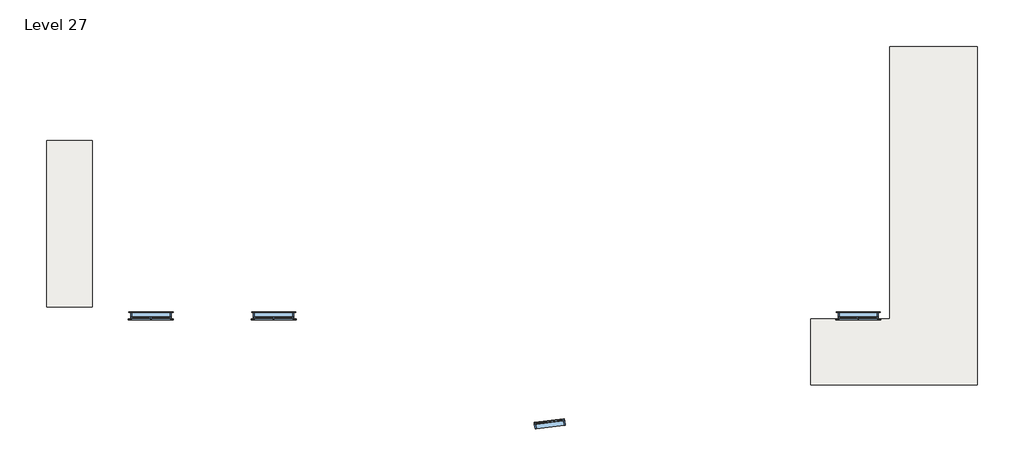
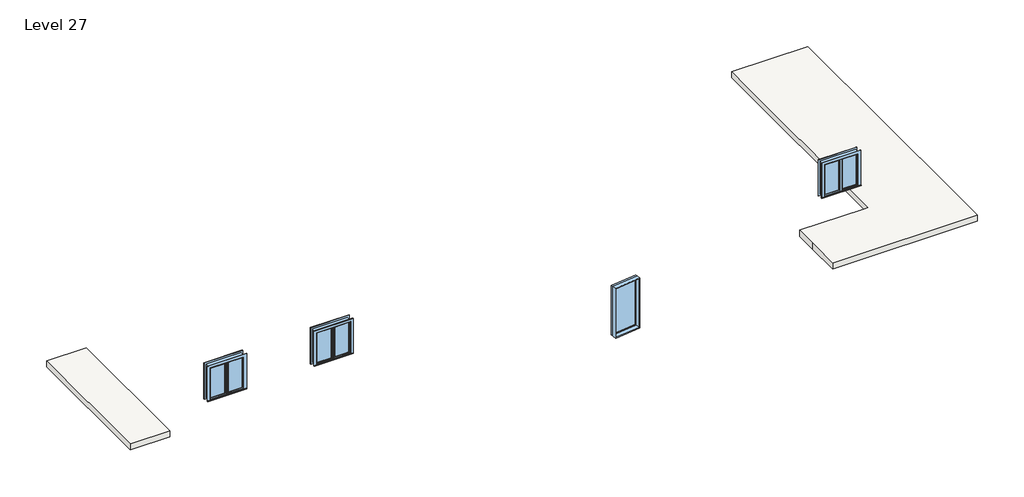
# One storey: 4 windows, 2 slabs.
"""IFC4 building model written with IfcOpenShell, lengths in millimetres."""

from ifc_helpers import new_model, si_unit, frame, origin, place, context, project, spatial, polyline, outline, extrude, transform, mapped, element, save
from components import window_0862ab64, window_9a779fa2

model = new_model("IFC4")

# Units and contexts
model_context = context("Model", 3, world=origin())
ifc_project = project(units=[si_unit("LENGTHUNIT", "METRE", prefix="MILLI")], contexts=[model_context])

# Site, building, storey
site = spatial("IfcSite", under=ifc_project)
building = spatial("IfcBuilding", under=site)
storey = spatial("IfcBuildingStorey", under=building, Name="Level 27", Elevation=42595.8)

# Slabs
placement = place(None, origin())
element("IfcSlab", 1, ObjectType="9\"", at=placement, inside=storey, context=model_context, shape_type="SweptSolid", body=[
    extrude(outline(polyline([(-17978.526008, -8690.0239591), (-16606.926008, -8690.0239591), (-16606.926008, -13719.2239591), (-17978.526008, -13719.2239591), (-17978.526008, -8690.0239591)])), frame((0.0, 0.0, 42367.2), z_axis=(0.0, 0.0, 1.0), x_axis=(1.0, 0.0, 0.0)), (0.0, 0.0, 1.0), 228.6),
])
element("IfcSlab", 2, ObjectType="9\"", at=placement, inside=storey, context=model_context, shape_type="SweptSolid", body=[
    extrude(outline(polyline([(5071.4396352, -14840.0808221), (5071.4396352, -14078.0808221), (7255.8396352, -14078.0808221), (7459.0396352, -14078.0808221), (7459.0396352, -5848.4808221), (10100.6396352, -5848.4808221), (10100.6396352, -14840.0808221), (10100.6396352, -16059.2808221), (5071.4396352, -16059.2808221), (5071.4396352, -14840.0808221)])), frame((0.0, 0.0, 42367.2), z_axis=(0.0, 0.0, 1.0), x_axis=(1.0, 0.0, 0.0)), (0.0, 0.0, 1.0), 228.6),
])

# Windows
window_shape = window_0862ab64(model_context)
element("IfcWindow", 3, ObjectType="Casement Dbl with Trim : 48\" x 48\"", at=placement, inside=storey, context=model_context, shape_type="MappedRepresentation", body=[
    mapped(window_shape, transform((-14829.9505427, -13957.4308221, 42595.8), x_axis=(-1.0, 0.0, 0.0), y_axis=(0.0, -1.0, 0.0), z_axis=(0.0, 0.0, 1.0))),
])
element("IfcWindow", 4, ObjectType="Casement Dbl with Trim : 48\" x 48\"", at=placement, inside=storey, context=model_context, shape_type="MappedRepresentation", body=[
    mapped(window_shape, transform((-11129.6382271, -13957.4308221, 42595.8), x_axis=(-1.0, 0.0, 0.0), y_axis=(0.0, -1.0, 0.0), z_axis=(0.0, 0.0, 1.0))),
])
element("IfcWindow", 5, ObjectType="Casement Dbl with Trim : 48\" x 48\"", at=placement, inside=storey, context=model_context, shape_type="MappedRepresentation", body=[
    mapped(window_shape, transform((6506.0494573, -13957.4308221, 42595.8), x_axis=(-1.0, 0.0, 0.0), y_axis=(0.0, -1.0, 0.0), z_axis=(0.0, 0.0, 1.0))),
])
window_2_shape = window_9a779fa2(model_context)
element("IfcWindow", 6, ObjectType="Fixed : 36\" x 72\"", at=placement, inside=storey, context=model_context, shape_type="MappedRepresentation", body=[
    mapped(window_2_shape, transform((-2764.84362, -17238.2448026, 43244.832135), x_axis=(0.9924631752743311, 0.12254324022316515, 0.0), y_axis=(-0.12254324022316515, 0.9924631752743311, 0.0), z_axis=(0.0, 0.0, 1.0))),
])

save(model, "model.ifc")

# Revit data of these elements
# Type "9\""
#   Assembly Code = "B1010"
#   Function = 0
#   Layers, outside or top first: 0' - 9" no material (function 1)
# Type "Casement Dbl with Trim : 48\" x 48\""
#   Type Mark = "10"
#   Construction Type Id = "GSP4R"
#   Assembly Code = "B2020100"
#   Analytic Construction = "1/8 in Pilkington single glazing"
#   Visual Light Transmittance = 0.9
#   Solar Heat Gain Coefficient = 0.78
#   Heat Transfer Coefficient (U) = 0.6496 BTU/(h·ft²·°F)
#   Height = 4' - 0"
#   Default Sill Height = 3' - 0"
#   Trim Projection - Ext. = 0' - 0 1/2"
#   Trim Projection - Int. = 0' - 0 3/4"
#   Trim Width - Exterior = 0' - 3 1/2"
#   Trim Width - Interior = 0' - 3 1/2"
#   Width = 4' - 0"
#   Window Inset = 0' - 0 3/4"
#   Define Thermal Properties by = 1
#   Glass Pane Material = Glass
#   Sash Material = Sash
#   Trim Exterior Material = Trim
#   Trim Interior Material = Trim
#   Wall Closure = (empty or 0)
# Type "Fixed : 36\" x 72\""
#   Type Mark = "9"
#   Construction Type Id = "GSP4R"
#   Assembly Code = "B2020100"
#   Analytic Construction = "1/8 in Pilkington single glazing"
#   Visual Light Transmittance = 0.9
#   Solar Heat Gain Coefficient = 0.78
#   Heat Transfer Coefficient (U) = 0.6496 BTU/(h·ft²·°F)
#   Height = 6' - 0"
#   Default Sill Height = 1' - 0"
#   Width = 3' - 0"
#   Window Inset = 0' - 0 3/4"
#   Define Thermal Properties by = 1
#   Glass Pane Material = Glass
#   Sash Material = Sash
#   Wall Closure = (empty or 0)
# Element 1 (IfcSlab, "9\"")
#   built-in parameter 1001955 = 3.14159 (stored number, unit not read)
#   Height Offset From Level = 0' - 0"
#   Phase Created = New Construction
#   Materials on its faces: "Default Floor"
# Element 2 (IfcSlab, "9\"")
#   built-in parameter 1001955 = -1.5708 (stored number, unit not read)
#   Height Offset From Level = 0' - 0"
#   Phase Created = New Construction
#   Materials on its faces: "Default Floor"
# Element 3 (IfcWindow, "Casement Dbl with Trim : 48\" x 48\"")
#   Mark = "21"
#   Phase Created = New Construction
#   Materials on its faces: "Sash", "Trim", "Glass"
# Element 4 (IfcWindow, "Casement Dbl with Trim : 48\" x 48\"")
#   Mark = "22"
#   Phase Created = New Construction
#   Materials on its faces: "Sash", "Trim", "Glass"
# Element 5 (IfcWindow, "Casement Dbl with Trim : 48\" x 48\"")
#   Mark = "48"
#   Phase Created = New Construction
#   Materials on its faces: "Sash", "Trim", "Glass"
# Element 6 (IfcWindow, "Fixed : 36\" x 72\"")
#   Mark = "3"
#   Phase Created = New Construction
#   Materials on its faces: "Sash", "Glass"
# Materials
#   "Glass": class "Glass", colour RGB 0 128 192, transparency 0.75, Description = "Soda Lime Glass", Cost = 0
#   "Sash": class "Wood", colour RGB 224 178 126, transparency 0
#   "Trim": class "Wood", colour RGB 224 178 126, transparency 0
#   "Default Floor": colour RGB 128 128 128, transparency 0
